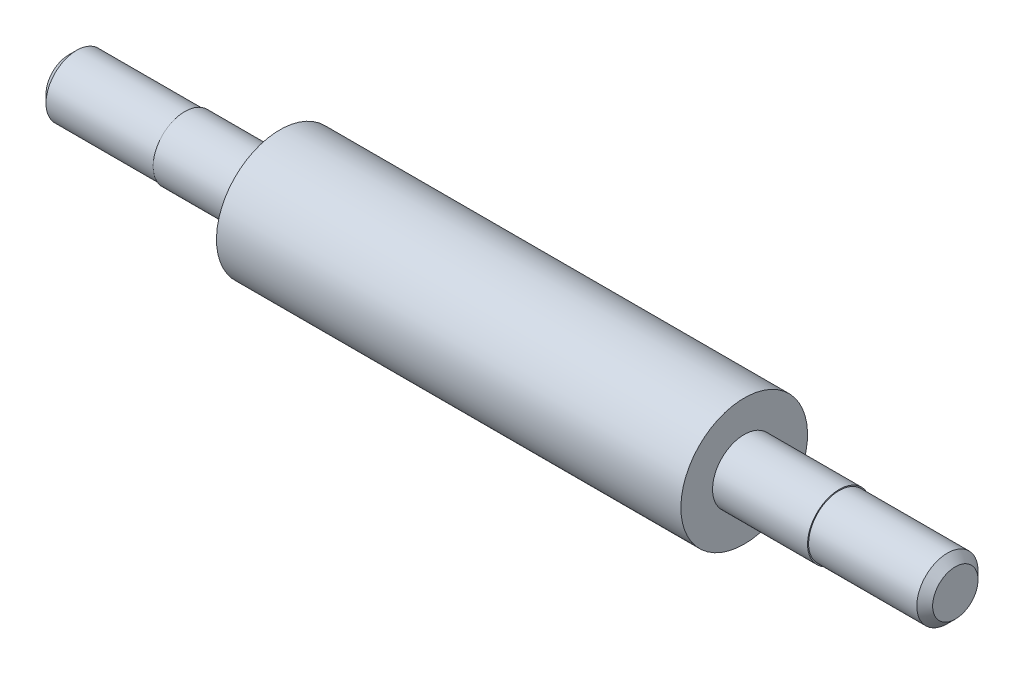
ISO-10303-21;
HEADER;
FILE_DESCRIPTION(('STEP AP214'),'2;1');
FILE_NAME('part.step','',(''),(''),'','','');
FILE_SCHEMA(('AUTOMOTIVE_DESIGN { 1 0 10303 214 1 1 1 1 }'));
ENDSEC;
DATA;
#1=APPLICATION_CONTEXT('core data for automotive mechanical design processes');
#2=APPLICATION_PROTOCOL_DEFINITION('international standard','automotive_design',2000,#1);
#3=PRODUCT_CONTEXT('',#1,'mechanical');
#4=PRODUCT('Part','Part','',(#3));
#5=PRODUCT_RELATED_PRODUCT_CATEGORY('part','',(#4));
#6=PRODUCT_DEFINITION_FORMATION('','',#4);
#7=PRODUCT_DEFINITION_CONTEXT('part definition',#1,'design');
#8=PRODUCT_DEFINITION('design','',#6,#7);
#9=PRODUCT_DEFINITION_SHAPE('','',#8);
#10=(LENGTH_UNIT() NAMED_UNIT(*) SI_UNIT(.MILLI.,.METRE.));
#11=(NAMED_UNIT(*) PLANE_ANGLE_UNIT() SI_UNIT($,.RADIAN.));
#12=(NAMED_UNIT(*) SI_UNIT($,.STERADIAN.) SOLID_ANGLE_UNIT());
#13=UNCERTAINTY_MEASURE_WITH_UNIT(LENGTH_MEASURE(1.E-05),#10,'distance_accuracy_value','');
#14=(GEOMETRIC_REPRESENTATION_CONTEXT(3) GLOBAL_UNCERTAINTY_ASSIGNED_CONTEXT((#13)) GLOBAL_UNIT_ASSIGNED_CONTEXT((#10,
#11,#12)) REPRESENTATION_CONTEXT('',''));
#15=CARTESIAN_POINT('',(0.,0.,0.));
#16=DIRECTION('',(0.,0.,1.));
#17=DIRECTION('',(1.,0.,0.));
#18=AXIS2_PLACEMENT_3D('',#15,#16,#17);
#19=CARTESIAN_POINT('',(220.,60.0000000000001,0.));
#20=DIRECTION('',(-1.,0.,0.));
#21=DIRECTION('',(0.,-1.,0.));
#22=AXIS2_PLACEMENT_3D('',#19,#20,#21);
#23=PLANE('',#22);
#24=CARTESIAN_POINT('',(220.,1.2050645439176E-13,0.));
#25=DIRECTION('',(-1.,0.,0.));
#26=DIRECTION('',(0.,-1.,0.));
#27=AXIS2_PLACEMENT_3D('',#24,#25,#26);
#28=CIRCLE('',#27,60.);
#29=CARTESIAN_POINT('',(220.,-59.9999999999999,0.));
#30=VERTEX_POINT('',#29);
#31=EDGE_CURVE('E82',#30,#30,#28,.T.);
#32=ORIENTED_EDGE('',*,*,#31,.F.);
#33=EDGE_LOOP('',(#32));
#34=FACE_BOUND('',#33,.T.);
#35=CARTESIAN_POINT('',(220.,1.2050645439176E-13,0.));
#36=DIRECTION('',(-1.,0.,0.));
#37=DIRECTION('',(0.,-1.,0.));
#38=AXIS2_PLACEMENT_3D('',#35,#36,#37);
#39=CIRCLE('',#38,29.9999999999999);
#40=CARTESIAN_POINT('',(220.,-29.9999999999997,0.));
#41=VERTEX_POINT('',#40);
#42=EDGE_CURVE('E58',#41,#41,#39,.T.);
#43=ORIENTED_EDGE('',*,*,#42,.T.);
#44=EDGE_LOOP('',(#43));
#45=FACE_BOUND('',#44,.T.);
#46=ADVANCED_FACE('F39',(#34,#45),#23,.F.);
#47=CARTESIAN_POINT('',(-420.,0.,0.));
#48=DIRECTION('',(-1.,0.,0.));
#49=DIRECTION('',(0.,-1.,0.));
#50=AXIS2_PLACEMENT_3D('',#47,#48,#49);
#51=CYLINDRICAL_SURFACE('',#50,29.9999999999999);
#52=ORIENTED_EDGE('',*,*,#42,.F.);
#53=EDGE_LOOP('',(#52));
#54=FACE_BOUND('',#53,.T.);
#55=CARTESIAN_POINT('',(310.,1.36694991996352E-13,0.));
#56=DIRECTION('',(-1.,0.,0.));
#57=DIRECTION('',(0.,-1.,0.));
#58=AXIS2_PLACEMENT_3D('',#55,#56,#57);
#59=CIRCLE('',#58,29.9999999999999);
#60=CARTESIAN_POINT('',(310.,-29.9999999999997,0.));
#61=VERTEX_POINT('',#60);
#62=EDGE_CURVE('E64',#61,#61,#59,.T.);
#63=ORIENTED_EDGE('',*,*,#62,.T.);
#64=EDGE_LOOP('',(#63));
#65=FACE_BOUND('',#64,.T.);
#66=ADVANCED_FACE('F88',(#54,#65),#51,.T.);
#67=CARTESIAN_POINT('',(310.,30.,0.));
#68=DIRECTION('',(-1.,0.,0.));
#69=DIRECTION('',(0.,-1.,0.));
#70=AXIS2_PLACEMENT_3D('',#67,#68,#69);
#71=PLANE('',#70);
#72=ORIENTED_EDGE('',*,*,#62,.F.);
#73=EDGE_LOOP('',(#72));
#74=FACE_BOUND('',#73,.T.);
#75=CARTESIAN_POINT('',(310.,1.36694991996352E-13,0.));
#76=DIRECTION('',(-1.,0.,0.));
#77=DIRECTION('',(0.,-1.,0.));
#78=AXIS2_PLACEMENT_3D('',#75,#76,#77);
#79=CIRCLE('',#78,28.9999999999998);
#80=CARTESIAN_POINT('',(310.,-28.9999999999997,0.));
#81=VERTEX_POINT('',#80);
#82=EDGE_CURVE('E69',#81,#81,#79,.T.);
#83=ORIENTED_EDGE('',*,*,#82,.T.);
#84=EDGE_LOOP('',(#83));
#85=FACE_BOUND('',#84,.T.);
#86=ADVANCED_FACE('F93',(#74,#85),#71,.F.);
#87=CARTESIAN_POINT('',(-420.,0.,0.));
#88=DIRECTION('',(-1.,0.,0.));
#89=DIRECTION('',(0.,-1.,0.));
#90=AXIS2_PLACEMENT_3D('',#87,#88,#89);
#91=CYLINDRICAL_SURFACE('',#90,28.9999999999998);
#92=CARTESIAN_POINT('',(412.5,1.55131937601583E-13,0.));
#93=DIRECTION('',(-1.,0.,0.));
#94=DIRECTION('',(0.,-1.,0.));
#95=AXIS2_PLACEMENT_3D('',#92,#93,#94);
#96=CIRCLE('',#95,28.9999999999998);
#97=CARTESIAN_POINT('',(412.5,-28.9999999999997,0.));
#98=VERTEX_POINT('',#97);
#99=EDGE_CURVE('E54',#98,#98,#96,.T.);
#100=ORIENTED_EDGE('',*,*,#99,.T.);
#101=EDGE_LOOP('',(#100));
#102=FACE_BOUND('',#101,.T.);
#103=ORIENTED_EDGE('',*,*,#82,.F.);
#104=EDGE_LOOP('',(#103));
#105=FACE_BOUND('',#104,.T.);
#106=ADVANCED_FACE('F103',(#102,#105),#91,.T.);
#107=CARTESIAN_POINT('',(420.,29.,0.));
#108=DIRECTION('',(-1.,0.,0.));
#109=DIRECTION('',(0.,-1.,0.));
#110=AXIS2_PLACEMENT_3D('',#107,#108,#109);
#111=PLANE('',#110);
#112=CARTESIAN_POINT('',(420.,1.56480982401966E-13,0.));
#113=DIRECTION('',(-1.,0.,0.));
#114=DIRECTION('',(0.,-1.,0.));
#115=AXIS2_PLACEMENT_3D('',#112,#113,#114);
#116=CIRCLE('',#115,21.4999999999998);
#117=CARTESIAN_POINT('',(420.,-21.4999999999996,0.));
#118=VERTEX_POINT('',#117);
#119=EDGE_CURVE('E51',#118,#118,#116,.F.);
#120=ORIENTED_EDGE('',*,*,#119,.T.);
#121=EDGE_LOOP('',(#120));
#122=FACE_BOUND('',#121,.T.);
#123=ADVANCED_FACE('F106',(#122),#111,.F.);
#124=CARTESIAN_POINT('',(-420.,29.,0.));
#125=DIRECTION('',(1.,0.,0.));
#126=DIRECTION('',(0.,1.,0.));
#127=AXIS2_PLACEMENT_3D('',#124,#125,#126);
#128=PLANE('',#127);
#129=CARTESIAN_POINT('',(-420.,0.,0.));
#130=DIRECTION('',(1.,0.,0.));
#131=DIRECTION('',(0.,1.,0.));
#132=AXIS2_PLACEMENT_3D('',#129,#130,#131);
#133=CIRCLE('',#132,21.4999999999996);
#134=CARTESIAN_POINT('',(-420.,21.4999999999996,0.));
#135=VERTEX_POINT('',#134);
#136=EDGE_CURVE('E50',#135,#135,#133,.F.);
#137=ORIENTED_EDGE('',*,*,#136,.T.);
#138=EDGE_LOOP('',(#137));
#139=FACE_BOUND('',#138,.T.);
#140=ADVANCED_FACE('F113',(#139),#128,.F.);
#141=CARTESIAN_POINT('',(-420.,0.,0.));
#142=DIRECTION('',(-1.,0.,0.));
#143=DIRECTION('',(0.,-1.,0.));
#144=AXIS2_PLACEMENT_3D('',#141,#142,#143);
#145=CYLINDRICAL_SURFACE('',#144,29.);
#146=CARTESIAN_POINT('',(-412.5,0.,0.));
#147=DIRECTION('',(1.,0.,0.));
#148=DIRECTION('',(0.,1.,0.));
#149=AXIS2_PLACEMENT_3D('',#146,#147,#148);
#150=CIRCLE('',#149,29.);
#151=CARTESIAN_POINT('',(-412.5,29.,0.));
#152=VERTEX_POINT('',#151);
#153=EDGE_CURVE('E10',#152,#152,#150,.T.);
#154=ORIENTED_EDGE('',*,*,#153,.T.);
#155=EDGE_LOOP('',(#154));
#156=FACE_BOUND('',#155,.T.);
#157=CARTESIAN_POINT('',(-310.,0.,0.));
#158=DIRECTION('',(-1.,0.,0.));
#159=DIRECTION('',(0.,-1.,0.));
#160=AXIS2_PLACEMENT_3D('',#157,#158,#159);
#161=CIRCLE('',#160,29.);
#162=CARTESIAN_POINT('',(-310.,-29.,0.));
#163=VERTEX_POINT('',#162);
#164=EDGE_CURVE('E68',#163,#163,#161,.T.);
#165=ORIENTED_EDGE('',*,*,#164,.T.);
#166=EDGE_LOOP('',(#165));
#167=FACE_BOUND('',#166,.T.);
#168=ADVANCED_FACE('F149',(#156,#167),#145,.T.);
#169=CARTESIAN_POINT('',(-310.,30.,0.));
#170=DIRECTION('',(1.,0.,0.));
#171=DIRECTION('',(0.,1.,0.));
#172=AXIS2_PLACEMENT_3D('',#169,#170,#171);
#173=PLANE('',#172);
#174=ORIENTED_EDGE('',*,*,#164,.F.);
#175=EDGE_LOOP('',(#174));
#176=FACE_BOUND('',#175,.T.);
#177=CARTESIAN_POINT('',(-310.,0.,0.));
#178=DIRECTION('',(-1.,0.,0.));
#179=DIRECTION('',(0.,-1.,0.));
#180=AXIS2_PLACEMENT_3D('',#177,#178,#179);
#181=CIRCLE('',#180,30.);
#182=CARTESIAN_POINT('',(-310.,-29.9999999999999,0.));
#183=VERTEX_POINT('',#182);
#184=EDGE_CURVE('E75',#183,#183,#181,.T.);
#185=ORIENTED_EDGE('',*,*,#184,.T.);
#186=EDGE_LOOP('',(#185));
#187=FACE_BOUND('',#186,.T.);
#188=ADVANCED_FACE('F144',(#176,#187),#173,.F.);
#189=CARTESIAN_POINT('',(-420.,0.,0.));
#190=DIRECTION('',(-1.,0.,0.));
#191=DIRECTION('',(0.,-1.,0.));
#192=AXIS2_PLACEMENT_3D('',#189,#190,#191);
#193=CYLINDRICAL_SURFACE('',#192,30.);
#194=ORIENTED_EDGE('',*,*,#184,.F.);
#195=EDGE_LOOP('',(#194));
#196=FACE_BOUND('',#195,.T.);
#197=CARTESIAN_POINT('',(-220.,0.,0.));
#198=DIRECTION('',(-1.,0.,0.));
#199=DIRECTION('',(0.,-1.,0.));
#200=AXIS2_PLACEMENT_3D('',#197,#198,#199);
#201=CIRCLE('',#200,30.);
#202=CARTESIAN_POINT('',(-220.,-29.9999999999999,0.));
#203=VERTEX_POINT('',#202);
#204=EDGE_CURVE('E73',#203,#203,#201,.T.);
#205=ORIENTED_EDGE('',*,*,#204,.T.);
#206=EDGE_LOOP('',(#205));
#207=FACE_BOUND('',#206,.T.);
#208=ADVANCED_FACE('F140',(#196,#207),#193,.T.);
#209=CARTESIAN_POINT('',(-220.,60.0000000000001,0.));
#210=DIRECTION('',(1.,0.,0.));
#211=DIRECTION('',(0.,1.,0.));
#212=AXIS2_PLACEMENT_3D('',#209,#210,#211);
#213=PLANE('',#212);
#214=ORIENTED_EDGE('',*,*,#204,.F.);
#215=EDGE_LOOP('',(#214));
#216=FACE_BOUND('',#215,.T.);
#217=CARTESIAN_POINT('',(-220.,0.,0.));
#218=DIRECTION('',(-1.,0.,0.));
#219=DIRECTION('',(0.,-1.,0.));
#220=AXIS2_PLACEMENT_3D('',#217,#218,#219);
#221=CIRCLE('',#220,60.);
#222=CARTESIAN_POINT('',(-220.,-60.,0.));
#223=VERTEX_POINT('',#222);
#224=EDGE_CURVE('E76',#223,#223,#221,.T.);
#225=ORIENTED_EDGE('',*,*,#224,.T.);
#226=EDGE_LOOP('',(#225));
#227=FACE_BOUND('',#226,.T.);
#228=ADVANCED_FACE('F129',(#216,#227),#213,.F.);
#229=CARTESIAN_POINT('',(-420.,0.,0.));
#230=DIRECTION('',(-1.,0.,0.));
#231=DIRECTION('',(0.,-1.,0.));
#232=AXIS2_PLACEMENT_3D('',#229,#230,#231);
#233=CYLINDRICAL_SURFACE('',#232,60.);
#234=ORIENTED_EDGE('',*,*,#224,.F.);
#235=EDGE_LOOP('',(#234));
#236=FACE_BOUND('',#235,.T.);
#237=ORIENTED_EDGE('',*,*,#31,.T.);
#238=EDGE_LOOP('',(#237));
#239=FACE_BOUND('',#238,.T.);
#240=ADVANCED_FACE('F83',(#236,#239),#233,.T.);
#241=CARTESIAN_POINT('',(412.5,1.55131937601583E-13,0.));
#242=DIRECTION('',(-1.,0.,0.));
#243=DIRECTION('',(0.,-1.,0.));
#244=AXIS2_PLACEMENT_3D('',#241,#242,#243);
#245=CONICAL_SURFACE('',#244,28.9999999999998,0.785398163397437);
#246=ORIENTED_EDGE('',*,*,#119,.F.);
#247=EDGE_LOOP('',(#246));
#248=FACE_BOUND('',#247,.T.);
#249=ORIENTED_EDGE('',*,*,#99,.F.);
#250=EDGE_LOOP('',(#249));
#251=FACE_BOUND('',#250,.T.);
#252=ADVANCED_FACE('F117',(#248,#251),#245,.T.);
#253=CARTESIAN_POINT('',(-420.,0.,0.));
#254=DIRECTION('',(1.,0.,0.));
#255=DIRECTION('',(0.,1.,0.));
#256=AXIS2_PLACEMENT_3D('',#253,#254,#255);
#257=CONICAL_SURFACE('',#256,21.4999999999996,0.78539816339745);
#258=ORIENTED_EDGE('',*,*,#153,.F.);
#259=EDGE_LOOP('',(#258));
#260=FACE_BOUND('',#259,.T.);
#261=ORIENTED_EDGE('',*,*,#136,.F.);
#262=EDGE_LOOP('',(#261));
#263=FACE_BOUND('',#262,.T.);
#264=ADVANCED_FACE('F45',(#260,#263),#257,.T.);
#265=CLOSED_SHELL('',(#46,#66,#86,#106,#123,#140,#168,#188,#208,#228,#240,#252,#264));
#266=MANIFOLD_SOLID_BREP('B2',#265);
#267=ADVANCED_BREP_SHAPE_REPRESENTATION('',(#18,#266),#14);
#268=SHAPE_DEFINITION_REPRESENTATION(#9,#267);
ENDSEC;
END-ISO-10303-21;
